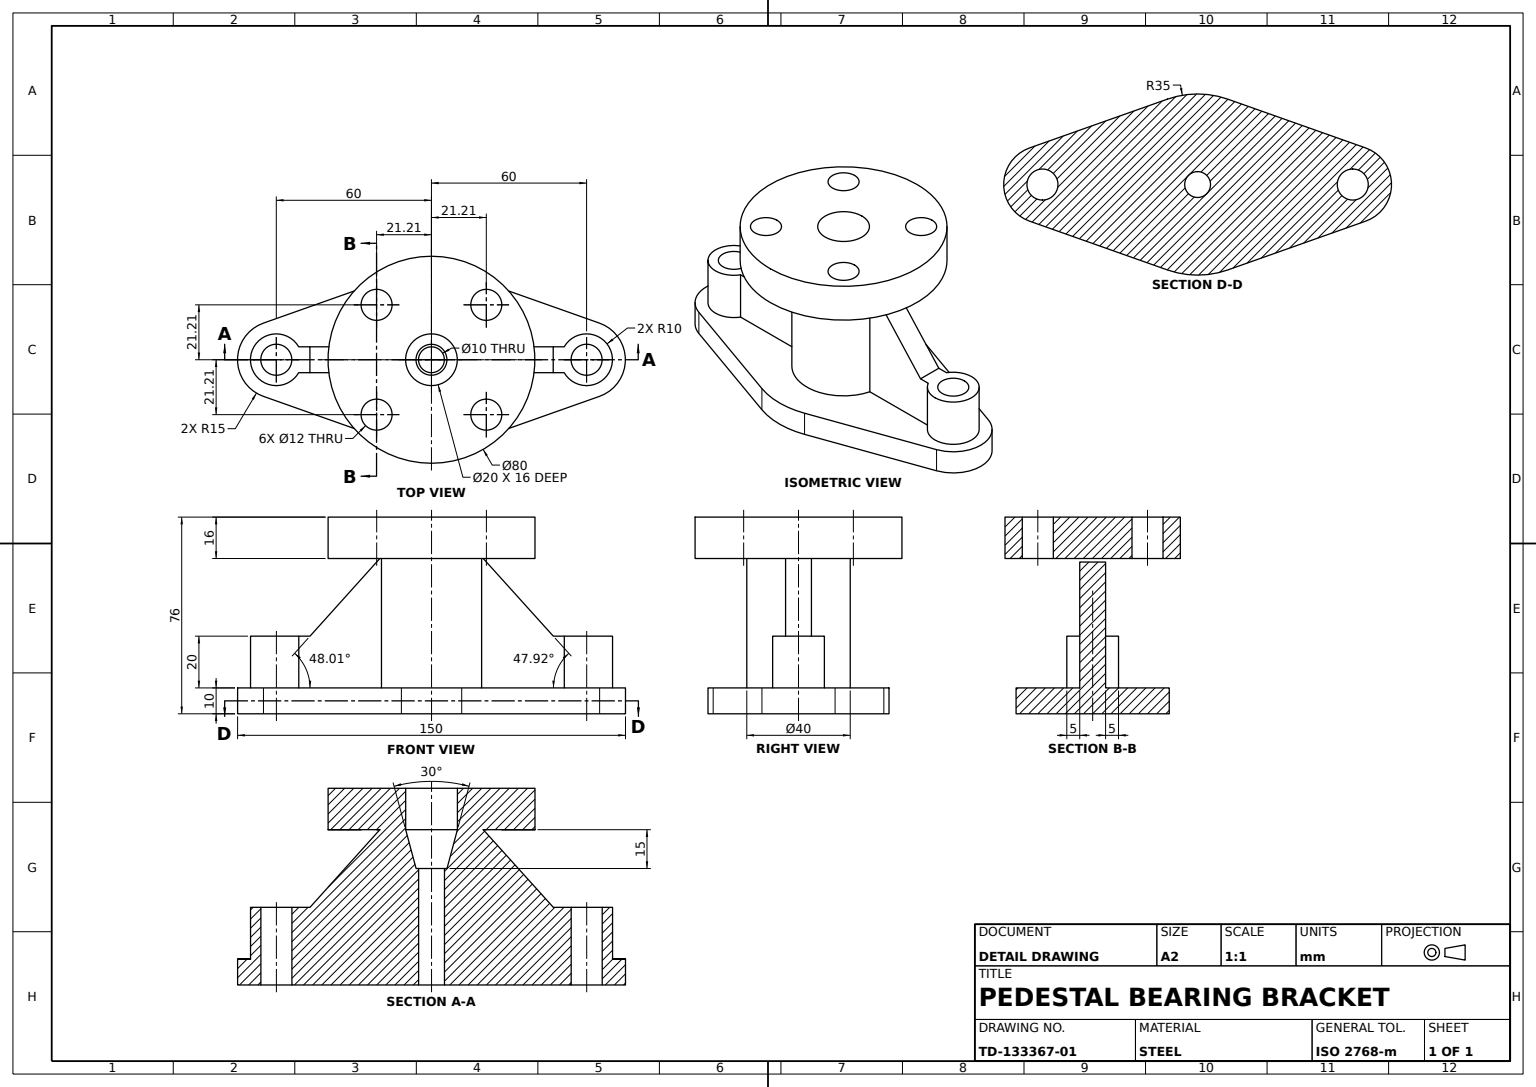
SolidWorks part; units mm, degrees
material "Plain Carbon Steel"
ref_plane "Front Plane" through (0, 0, 0) normal (0, 0, 1) x (1, 0, 0)
ref_plane "Top Plane" through (0, 0, 0) normal (0, 1, 0) x (1, 0, 0)
ref_plane "Right Plane" through (0, 0, 0) normal (1, 0, 0) x (0, 0, -1)
sketch "Base Flange Sketch" plane through (0, 0, 0) normal (0, 1, 0) x (1, 0, 0)
  line L0 (-11.6667, 32.9983) -> (-65, 14.1421)
  line L1 (11.6667, 32.9983) -> (65, 14.1421)
  line L2 (-65, -14.1421) -> (-11.6667, -32.9983)
  line L3 (11.6667, -32.9983) -> (65, -14.1421)
  arc A0 (-11.6667, -32.9983) -> (11.6667, -32.9983) centre (0, 0) ccw
  circle A1 centre (0, 0) radius 5
  arc A2 (-65, 14.1421) -> (-65, -14.1421) centre (-60, 0) ccw
  circle A3 centre (-60, 0) radius 6
  circle A4 centre (60, 0) radius 6
  arc A5 (65, -14.1421) -> (65, 14.1421) centre (60, 0) ccw
  arc A6 (11.6667, 32.9983) -> (-11.6667, 32.9983) centre (0, 0) ccw
  dimension "D1" = 12
  dimension "D2" = 12
  dimension "D5" = 70
  dimension "D6" = 10
  dimension "D7" = 30
  dimension "D8" = 30
  dimension "D3" = 60
  dimension "D4" = 60
extrude "Base Flange" add sketch "Base Flange Sketch" along normal blind 10
sketch "Pillar and Lug Bosses Sketch" plane through (0, 10, 0) normal (0, 1, 0) x (1, 0, 0)
  circle A0 centre (0, 0) radius 5
  circle A1 centre (0, 0) radius 20
  circle A2 centre (-60, 0) radius 6
  circle A3 centre (-60, 0) radius 10
  circle A4 centre (60, 0) radius 6
  circle A5 centre (60, 0) radius 10
  dimension "D1" = 20
  dimension "D2" = 20
  dimension "D3" = 12
  dimension "D4" = 12
  dimension "D5" = 10
  dimension "D6" = 40
extrude "Pillar and Lug Bosses" add sketch "Pillar and Lug Bosses Sketch" along normal blind 20
sketch "Upper Pillar Sketch" plane through (0, 30, 0) normal (0, 1, 0) x (1, 0, 0)
  circle A0 centre (0, 0) radius 5
  circle A1 centre (0, 0) radius 20
  dimension "D1" = 10
  dimension "D2" = 40
extrude "Upper Pillar Ø40" add sketch "Upper Pillar Sketch" along normal blind 30
ref_plane "Web Plane" through (0, 0, 0) normal (0, 0, 1) x (1, 0, 0)
sketch "Support Web Sketch" plane through (0, 0, 0) normal (0, 0, 1) x (1, 0, 0)
  line L0 (-47, 30) -> (-52, 30)
  line L1 (-47, 30) -> (-20, 60)
  line L2 (52.0908, 30) -> (47.0908, 30)
  line L3 (70, 30) -> (50, 30) construction
  line L4 (47.0908, 30) -> (20, 60)
  line L5 (-50, 30) -> (-70, 30) construction
  line L7 (-52, 30) -> (-52, 10)
  line L8 (-65, 10) -> (-11.6667, 10) construction
  line L9 (-52, 10) -> (-16.5687, 10)
  line L10 (-16.5687, 10) -> (-16.5687, 60)
  line L11 (20, 60) -> (-20, 60) construction
  line L12 (-16.5687, 60) -> (-20, 60)
  line L13 (20, 60) -> (17.3522, 60)
  line L14 (17.3522, 60) -> (17.3522, 10)
  line L15 (11.6667, 10) -> (65, 10) construction
  line L16 (17.3522, 10) -> (52.0908, 10)
  line L17 (52.0908, 10) -> (52.0908, 30)
  dimension "D1" = 5
  dimension "D2" = 30
  dimension "D3" = 27.0908
  dimension "D4" = 17.3522
  dimension "D5" = 16.5687
  dimension "D6" = 35.4313
  dimension "D7" = 34.7386
extrude "Support Web" add sketch "Support Web Sketch" along normal mid plane 10
sketch "Tapered Bore Sketch" plane through (0, 60, 0) normal (0, 1, 0) x (1, 0, 0)
  circle A0 centre (0, 0) radius 10
  dimension "D1" = 20
extrude "Tapered Bore Ø20" cut sketch "Tapered Bore Sketch" against normal blind 15 draft 15
sketch "Top Flange Sketch" plane through (0, 60, 0) normal (0, 1, 0) x (1, 0, 0)
  circle A0 centre (0, 0) radius 40
  circle A1 centre (0, 0) radius 10
  circle A3 centre (21.2132, 21.2132) radius 6
  circle A4 centre (21.2132, -21.2132) radius 6
  circle A5 centre (-21.2132, -21.2132) radius 6
  circle A6 centre (-21.2132, 21.2132) radius 6
  dimension "D1" = 20
  dimension "D2" = 80
  dimension "D4" = 21.2132
  dimension "D5" = 12
  dimension "D3" = 30
  dimension "D6" = 4
  dimension "D7" = 30
  dimension "D8" = 21.2132
extrude "Top Flange Ø80 with Holes 4xØ12" add sketch "Top Flange Sketch" along normal blind 16
